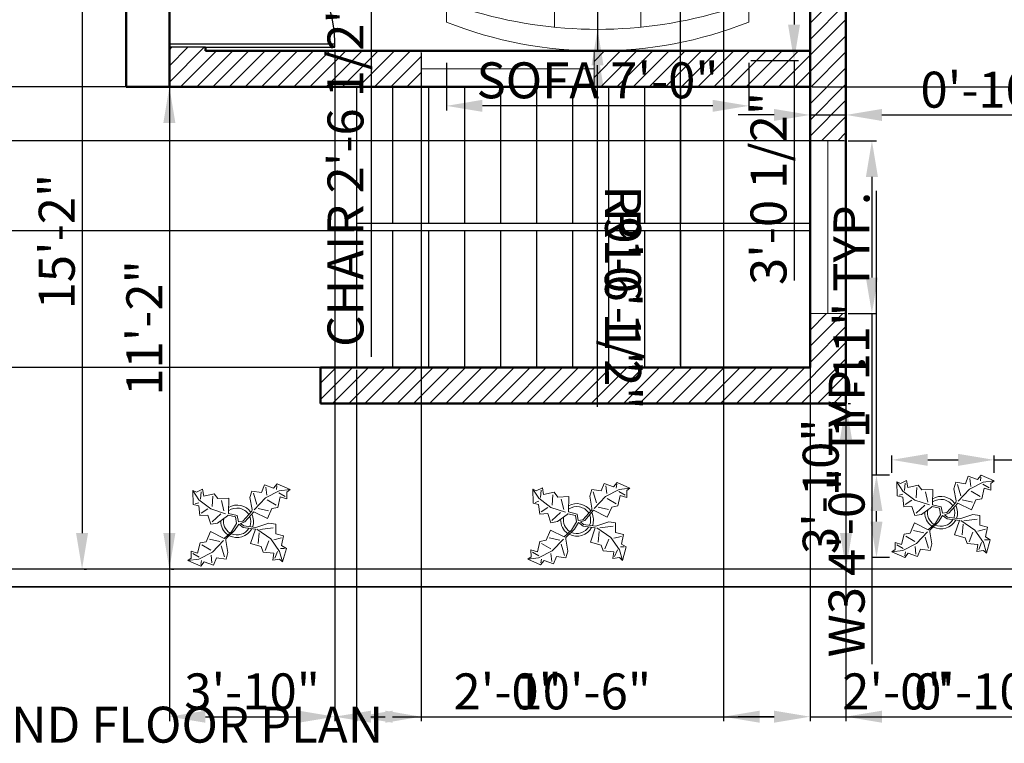
# Model space of a CAD drawing. Units: inches. Extents: x 2206 to 2843, y 1750 to 2489.
# Tile 2 of 8: x 2428 to 2702, y 1751 to 1953. Entities that reach past the tile are written whole.
import ezdxf

# ---------------------------------------------------------------- set-up
doc = ezdxf.new("R2010")
doc.units = ezdxf.units.IN
for name, color, linetype, lineweight in [('A-ANNO-DIMS', 2, 'Continuous', 18), ('A-ANNO-TEXT', 7, 'Continuous', 25), ('A-DOOR', 3, 'Continuous', 25), ('A-FLOR-STRS', 7, 'Continuous', 25), ('A-FURN', 21, 'Continuous', 18), ('A-GLAZ', 4, 'Continuous', 18), ('A-WALL', 7, 'Continuous', 50), ('A-WALL-PATT', 252, 'Continuous', 13), ('C-PROP', 7, 'Continuous', 35), ('L-PLNT', 92, 'Continuous', 18), ('L-SITE-WALL', 8, 'Continuous', 25)]:
    doc.layers.add(name, color=color, linetype=linetype, lineweight=lineweight)
doc.styles.get("Standard").update_dxf_attribs({"font": 'arial.ttf'})
doc.dimstyles.new('ISO-25', dxfattribs={"dimtxt": 10, "dimasz": 10, "dimexe": 1.25, "dimexo": 0.625, "dimtad": 1, "dimdec": 1, "dimlunit": 3, "dimtxsty": 'Standard', "dimcen": 2.5, "dimadec": 0, "dimazin": 0, "dimtfac": 1, "dimtdec": 1, "dimtmove": 0, "dimatfit": 3, "dimfxl": 1, "dimarcsym": 0})

# ---------------------------------------------------------------- blocks, each defined once
blk = doc.blocks.new('Sofa - Roundback 7 ft.')
for p, q in [((-12.00002, -32.4421), (-12.00003, -6.5971)), ((11.99997, -32.4421), (11.99998, -6.5971)), ((-36.000027, -34), (-36.000027, -11.4696)), ((-35.999844, -13.3819), (35.9998, -13.3819)), ((35.99998, -34), (35.99998, -11.4696)), ((-36.000027, -32.4421), (35.99998, -32.4421))]:
    blk.add_line(p, q)
for points in [[(-36.000027, -34), (-42.000027, -34), (-42.000027, -8)], [(41.99998, -8), (41.99998, -34), (35.99998, -34)]]:
    blk.add_lwpolyline(points)
for centre, radius, start, end in [((0, -114.25), 114.25, 68.43141, 111.5686), ((-0.00001, -127.1968), 121.1968, 72.72033, 107.2797)]:
    blk.add_arc(centre, radius, start, end)
blk = doc.blocks.new('Plant - Rubber or Philodendron')
for p, q in [((-16.2005, 11.4774), (-13.9899, 8.1064)), ((-16.2005, 11.4774), (-14.8639, 10.7964)), ((-16.0159, 6.3329), (-16.2005, 11.4774)), ((-14.8639, 10.7964), (-12.6195, 11.8975)), ((-13.3174, 8.325), (-13.0735, 11.0065)), ((-12.6195, 11.8975), (-12.1909, 9.4345)), ((4.6914, 8.8812), (5.3859, 11.2828)), ((5.3859, 11.2828), (8.8871, 10.7908)), ((8.8871, 10.7908), (9.9809, 13.4933)), ((9.9809, 13.4933), (13.3837, 12.301)), ((15.3859, 11.3055), (10.3916, 8.7942)), ((10.5828, 12.6946), (10.8893, 9.7953)), ((13.3837, 12.301), (14.68, 13.9039)), ((14.5816, 13.2037), (14.3848, 11.8033)), ((14.68, 13.9039), (19.3848, 11.8146)), ((19.3848, 11.8146), (15.3859, 11.3055)), ((19.3848, 11.8146), (18.1868, 10.9119)), ((18.1868, 10.9119), (18.1925, 8.4119)), ((-13.9899, 8.1064), (-9.5434, 4.7185)), ((-12.1909, 9.4345), (-8.3829, 10.3)), ((-8.8369, 9.409), (-9.0894, 5.6095)), ((-8.3829, 10.3), (-7.0549, 8.501)), ((-7.0549, 8.501), (-3.0284, 8.6941)), ((-4.8529, 4.012), (-5.7184, 7.82)), ((-3.0284, 8.6941), (-3.0709, 3.1041)), ((4.6914, 8.8812), (5.5014, 4.4831)), ((5.9878, 10.4842), (7.1971, 6.3869)), ((10.3916, 8.7942), (6.2847, 4.4028)), ((14.2977, 6.1031), (10.9934, 7.9956)), ((15.7909, 9.1065), (14.8995, 5.3044)), ((15.2875, 10.6053), (17.5907, 9.2105)), ((18.1925, 8.4119), (15.7909, 9.1065)), ((-14.0069, 5.8704), (-16.0159, 6.3329)), ((-15.3434, 6.5514), (-13.9984, 6.9884)), ((-13.5868, 2.2894), (-14.0069, 5.8704)), ((-13.1329, 3.1804), (-10.6614, 4.727)), ((-9.5434, 4.7185), (-4.1917, 2.9888)), ((2.1141, 0.2298), (5.4346, 3.9146)), ((6.1032, 3.6844), (2.8262, -0.031)), ((5.4346, 3.9146), (5.5014, 4.4831)), ((11.1089, 1.1958), (6.1032, 3.6844)), ((7.7005, 4.8881), (11.5025, 3.9967)), ((12.7005, 4.8994), (11.1089, 1.1958)), ((14.8995, 5.3044), (12.7005, 4.8994)), ((-10.6784, 2.491), (-13.5868, 2.2894)), ((-9.5858, -0.8715), (-10.6784, 2.491)), ((-9.1318, 0.0195), (-5.9793, 2.9025)), ((-7.1228, -0.443), (-3.5248, 2.2131)), ((-3.5248, 2.2131), (-3.3011, 2.4355)), ((-3.3011, 2.4355), (-0.5306, 1.7947)), ((-3.0709, 3.1041), (0.0797, 2.3163)), ((-0.5306, 1.7947), (-0.2255, -0.5527)), ((-0.5306, 1.7947), (-0.5306, 1.7947)), ((0.0797, 2.3163), (0.4866, -0.031)), ((0.4866, -0.031), (2.1141, 0.2298)), ((-11.3237, -7.2629), (-9.7321, -3.5593)), ((-9.7321, -3.5593), (-4.7264, -6.0479)), ((-7.1228, -0.443), (-9.5858, -0.8715)), ((-4.0579, -6.2781), (-0.9375, -3.1608)), ((-2.019, -3.6148), (-0.2255, -0.5527)), ((-0.9375, -3.1608), (0.5883, -0.8135)), ((0.5883, -0.8135), (2.2447, -2.0916)), ((2.8262, -0.031), (1.3003, -0.5527)), ((1.3003, -0.5527), (2.4193, -1.4655)), ((2.2447, -2.0916), (6.7108, -2.6626)), ((2.4193, -1.4655), (6.895, -2.1175)), ((4.943, -7.9659), (6.7108, -2.6626)), ((11.6605, -0.5413), (6.895, -2.1175)), ((12.3677, -6.1981), (7.219, -2.6772)), ((8.3544, -2.7453), (13.1973, -2.1704)), ((11.6605, -0.5413), (14.1354, -0.8948)), ((14.1354, -0.8948), (14.1354, -4.4304)), ((-6.3237, -7.2516), (-10.1257, -6.3602)), ((-9.0148, -11.1577), (-4.9047, -6.8122)), ((-2.019, -3.6148), (-4.7264, -6.0479)), ((-4.1246, -6.8466), (-4.0579, -6.2781)), ((-3.3146, -11.2447), (-4.1246, -6.8466)), ((8.125, -4.0768), (7.7715, -7.9659)), ((10.2463, -10.4408), (11.6605, -6.9053)), ((15.5496, -10.7943), (12.3677, -6.1981)), ((16.2567, -5.8446), (13.4283, -6.5517)), ((14.1354, -4.4304), (16.9638, -5.1375)), ((16.9638, -5.1375), (16.2567, -8.673)), ((-16.8157, -10.7754), (-14.4141, -11.4699)), ((-16.8101, -13.2754), (-16.8157, -10.7754)), ((-14.4141, -11.4699), (-13.5228, -7.6679)), ((-13.5228, -7.6679), (-11.3237, -7.2629)), ((-12.921, -8.4665), (-9.6166, -10.359)), ((-4.611, -12.8477), (-5.8203, -8.7504)), ((8.8321, -9.0266), (4.943, -7.9659)), ((9.5392, -11.1479), (8.8321, -9.0266)), ((14.8425, -10.7943), (13.7819, -13.2692)), ((16.6103, -14.6834), (15.5496, -10.7943)), ((17.3174, -9.7337), (15.9032, -9.7337)), ((16.2567, -8.673), (18.0245, -9.7337)), ((18.0245, -9.7337), (16.6103, -14.6834)), ((-18.008, -14.1781), (-16.8101, -13.2754)), ((-18.008, -14.1781), (-14.0091, -13.669)), ((-13.3032, -16.2674), (-18.008, -14.1781)), ((-13.9107, -12.9688), (-16.2139, -11.574)), ((-14.0091, -13.669), (-9.0148, -11.1577)), ((-13.2048, -15.5672), (-13.008, -14.1668)), ((-9.206, -15.0581), (-9.5126, -12.1588)), ((-7.5103, -13.1543), (-8.6042, -15.8568)), ((-4.0092, -13.6463), (-7.5103, -13.1543)), ((-3.3146, -11.2447), (-4.0092, -13.6463)), ((13.4283, -11.5015), (9.5392, -11.1479)), ((13.0748, -13.9763), (13.4283, -11.5015)), ((15.5496, -13.6228), (13.0748, -13.9763)), ((16.6103, -14.6834), (15.5496, -13.6228)), ((-12.0069, -14.6645), (-13.3032, -16.2674)), ((-8.6042, -15.8568), (-12.0069, -14.6645))]:
    blk.add_line(p, q)
for centre, radius, start, end in [((0, 0), 6.1275, 34.37569, 120.1028), ((-0.0601, -0.2075), 5.2461, 33.82192, 124.9414), ((0.0308, 0.1664), 6, 178.6147, 235.1169), ((0.0308, 0.1664), 5, 168.1647, 238.6725), ((-0.2664, 0.1682), 5.2775, 338.4094, 20.03007), ((-0.098, 0.1364), 6.1288, 341.2017, 26.09184), ((-0.0234, 0.3825), 6.1492, 242.5812, 331.2714), ((-0.1102, 0.4886), 5.2883, 247.3711, 327.472)]:
    blk.add_arc(centre, radius, start, end)
blk = doc.blocks.new('*D16')
at = {"layer": 'A-ANNO-DIMS', "color": 0, "lineweight": -2, "transparency": 16777216}
for p, q in [((2470.2, 1933.9), (2470.83, 1933.9)), ((2469.58, 1923.9), (2469.58, 1809.9)), ((2470.2, 1799.9), (2470.83, 1799.9))]:
    blk.add_line(p, q, dxfattribs=at)
at = {"layer": 'A-ANNO-DIMS', "color": 0, "transparency": 16777216}
for points in [[(2467.91, 1923.9), (2471.25, 1923.9), (2469.58, 1933.9)], [(2467.91, 1809.9), (2471.25, 1809.9), (2469.58, 1799.9)]]:
    blk.add_solid(points, dxfattribs=at)
at = {"layer": 'Defpoints', "color": 0, "transparency": 16777216}
for p in [(2469.58, 1933.9), (2469.58, 1799.9), (2469.58, 1799.9)]:
    blk.add_point(p, dxfattribs=at)
at = {"layer": 'A-ANNO-DIMS', "color": 0, "transparency": 16777216, "insert": (2463.93, 1866.9), "char_height": 10, "attachment_point": 5, "rotation": 90}
blk.add_mtext('11\'-2"', dxfattribs=at)
blk = doc.blocks.new('*D18')
at = {"layer": 'A-ANNO-DIMS', "color": 0, "lineweight": -2, "transparency": 16777216}
for p, q in [((2445.95, 1981.9), (2446.57, 1981.9)), ((2445.32, 1971.9), (2445.32, 1809.9)), ((2445.95, 1799.9), (2446.57, 1799.9))]:
    blk.add_line(p, q, dxfattribs=at)
at = {"layer": 'A-ANNO-DIMS', "color": 0, "transparency": 16777216}
for points in [[(2443.65, 1971.9), (2446.99, 1971.9), (2445.32, 1981.9)], [(2443.65, 1809.9), (2446.99, 1809.9), (2445.32, 1799.9)]]:
    blk.add_solid(points, dxfattribs=at)
at = {"layer": 'Defpoints', "color": 0, "transparency": 16777216}
for p in [(2445.32, 1981.9), (2445.32, 1799.9), (2445.32, 1799.9)]:
    blk.add_point(p, dxfattribs=at)
at = {"layer": 'A-ANNO-DIMS', "color": 0, "transparency": 16777216, "insert": (2439.59, 1890.9), "char_height": 10, "attachment_point": 5, "rotation": 90}
blk.add_mtext('15\'-2"', dxfattribs=at)
blk = doc.blocks.new('*D19')
at = {"layer": 'A-ANNO-DIMS', "color": 0, "lineweight": -2, "transparency": 16777216}
for p, q in [((2658.2, 1845.9), (2658.83, 1845.9)), ((2657.58, 1835.9), (2657.58, 1809.9)), ((2658.2, 1799.9), (2658.83, 1799.9))]:
    blk.add_line(p, q, dxfattribs=at)
at = {"layer": 'A-ANNO-DIMS', "color": 0, "transparency": 16777216}
for points in [[(2655.91, 1835.9), (2659.25, 1835.9), (2657.58, 1845.9)], [(2655.91, 1809.9), (2659.25, 1809.9), (2657.58, 1799.9)]]:
    blk.add_solid(points, dxfattribs=at)
at = {"layer": 'Defpoints', "color": 0, "transparency": 16777216}
for p in [(2657.58, 1845.9), (2657.58, 1799.9), (2657.58, 1799.9)]:
    blk.add_point(p, dxfattribs=at)
at = {"layer": 'A-ANNO-DIMS', "color": 0, "transparency": 16777216, "insert": (2651.85, 1822.9), "char_height": 10, "attachment_point": 5, "rotation": 90}
blk.add_mtext('3\'-10"', dxfattribs=at)
blk = doc.blocks.new('WIN-48IN')
for p, q in [((0, 10), (0, 0)), ((48, 10), (48, 0)), ((48, 5), (0, 5))]:
    blk.add_line(p, q)
blk = doc.blocks.new('*D27')
at = {"layer": 'A-ANNO-DIMS', "color": 0, "lineweight": -2, "transparency": 16777216}
for p, q in [((2670.31, 1826.6), (2670.31, 1831.49)), ((2680.31, 1830.24), (2688.72, 1830.24)), ((2698.72, 1826.6), (2698.72, 1831.49)), ((2698.72, 1830.24), (2842.63, 1830.24))]:
    blk.add_line(p, q, dxfattribs=at)
at = {"layer": 'A-ANNO-DIMS', "color": 0, "transparency": 16777216}
for points in [[(2680.31, 1831.91), (2680.31, 1828.57), (2670.31, 1830.24)], [(2688.72, 1831.91), (2688.72, 1828.57), (2698.72, 1830.24)]]:
    blk.add_solid(points, dxfattribs=at)
at = {"layer": 'Defpoints', "color": 0, "transparency": 16777216}
for p in [(2698.72, 1830.24), (2670.31, 1825.98), (2698.72, 1825.98)]:
    blk.add_point(p, dxfattribs=at)
at = {"layer": 'A-ANNO-DIMS', "color": 0, "transparency": 16777216, "insert": (2775.67, 1836.03), "char_height": 10, "attachment_point": 5}
blk.add_mtext('PLANT 2\'-4 1/2" TYP.', dxfattribs=at)
blk = doc.blocks.new('*D28')
at = {"layer": 'A-ANNO-DIMS', "color": 0, "lineweight": -2, "transparency": 16777216}
for p, q in [((2666.05, 1825.98), (2666.05, 1905.01)), ((2669.69, 1825.98), (2664.8, 1825.98)), ((2666.05, 1813.06), (2666.05, 1815.98)), ((2669.69, 1803.06), (2664.8, 1803.06))]:
    blk.add_line(p, q, dxfattribs=at)
at = {"layer": 'A-ANNO-DIMS', "color": 0, "transparency": 16777216}
for points in [[(2664.38, 1815.98), (2667.72, 1815.98), (2666.05, 1825.98)], [(2664.38, 1813.06), (2667.72, 1813.06), (2666.05, 1803.06)]]:
    blk.add_solid(points, dxfattribs=at)
at = {"layer": 'Defpoints', "color": 0, "transparency": 16777216}
for p in [(2666.05, 1825.98), (2670.31, 1825.98), (2670.31, 1803.06)]:
    blk.add_point(p, dxfattribs=at)
at = {"layer": 'A-ANNO-DIMS', "color": 0, "transparency": 16777216, "insert": (2660.4, 1870.5), "char_height": 10, "attachment_point": 5, "rotation": 90}
blk.add_mtext('1\'-11" TYP.', dxfattribs=at)
blk = doc.blocks.new('*D39')
at = {"layer": 'A-ANNO-DIMS', "color": 0, "lineweight": -2, "transparency": 16777216}
for p, q in [((2658.2, 1918.9), (2666.03, 1918.9)), ((2664.78, 1908.9), (2664.78, 1880.9)), ((2658.2, 1870.9), (2666.03, 1870.9)), ((2664.78, 1870.9), (2664.78, 1773.45))]:
    blk.add_line(p, q, dxfattribs=at)
at = {"layer": 'A-ANNO-DIMS', "color": 0, "transparency": 16777216}
for points in [[(2663.11, 1908.9), (2666.45, 1908.9), (2664.78, 1918.9)], [(2663.11, 1880.9), (2666.45, 1880.9), (2664.78, 1870.9)]]:
    blk.add_solid(points, dxfattribs=at)
at = {"layer": 'Defpoints', "color": 0, "transparency": 16777216}
for p in [(2657.58, 1918.9), (2657.58, 1870.9), (2664.78, 1870.9)]:
    blk.add_point(p, dxfattribs=at)
at = {"layer": 'A-ANNO-DIMS', "color": 0, "transparency": 16777216, "insert": (2659.05, 1817.17), "char_height": 10, "attachment_point": 5, "rotation": 90}
blk.add_mtext('W3 4\'-0" TYP.', dxfattribs=at)
blk = doc.blocks.new('*D40')
at = {"layer": 'A-ANNO-DIMS', "color": 0, "lineweight": -2, "transparency": 16777216}
for p, q in [((2637.58, 1926.1), (2627.58, 1926.1)), ((2647.58, 1919.52), (2647.58, 1927.35)), ((2647.58, 1926.1), (2657.58, 1926.1)), ((2657.58, 1919.52), (2657.58, 1927.35)), ((2667.58, 1926.1), (2747.55, 1926.1))]:
    blk.add_line(p, q, dxfattribs=at)
at = {"layer": 'A-ANNO-DIMS', "color": 0, "transparency": 16777216}
for points in [[(2637.58, 1927.77), (2637.58, 1924.43), (2647.58, 1926.1)], [(2667.58, 1927.77), (2667.58, 1924.43), (2657.58, 1926.1)]]:
    blk.add_solid(points, dxfattribs=at)
at = {"layer": 'Defpoints', "color": 0, "transparency": 16777216}
for p in [(2657.58, 1926.1), (2647.58, 1918.9), (2657.58, 1918.9)]:
    blk.add_point(p, dxfattribs=at)
at = {"layer": 'A-ANNO-DIMS', "color": 0, "transparency": 16777216, "insert": (2712.57, 1931.83), "char_height": 10, "attachment_point": 5}
blk.add_mtext('0\'-10" TYP.', dxfattribs=at)
blk = doc.blocks.new('*D45')
at = {"layer": 'A-ANNO-DIMS', "color": 0, "lineweight": -2, "transparency": 16777216}
for p, q in [((2529.57, 2032.2), (2524.36, 2032.2)), ((2525.61, 2022.2), (2525.61, 2011.61)), ((2529.57, 2001.61), (2524.36, 2001.61)), ((2525.61, 2001.61), (2525.61, 1858.87))]:
    blk.add_line(p, q, dxfattribs=at)
at = {"layer": 'A-ANNO-DIMS', "color": 0, "transparency": 16777216}
for points in [[(2523.94, 2022.2), (2527.27, 2022.2), (2525.61, 2032.2)], [(2523.94, 2011.61), (2527.27, 2011.61), (2525.61, 2001.61)]]:
    blk.add_solid(points, dxfattribs=at)
at = {"layer": 'Defpoints', "color": 0, "transparency": 16777216}
for p in [(2530.19, 2032.2), (2525.61, 2001.61), (2530.19, 2001.61)]:
    blk.add_point(p, dxfattribs=at)
at = {"layer": 'A-ANNO-DIMS', "color": 0, "transparency": 16777216, "insert": (2519.81, 1925.24), "char_height": 10, "attachment_point": 5, "rotation": 90}
blk.add_mtext('CHAIR 2\'-6 1/2" TYP.', dxfattribs=at)
blk = doc.blocks.new('*D51')
at = {"layer": 'A-ANNO-DIMS', "color": 0, "lineweight": -2, "transparency": 16777216}
for p, q in [((2546.55, 1940.61), (2546.55, 1927.38)), ((2630.55, 1940.61), (2630.55, 1927.38)), ((2620.55, 1928.63), (2556.55, 1928.63))]:
    blk.add_line(p, q, dxfattribs=at)
at = {"layer": 'A-ANNO-DIMS', "color": 0, "transparency": 16777216}
for points in [[(2556.55, 1930.3), (2556.55, 1926.97), (2546.55, 1928.63)], [(2620.55, 1930.3), (2620.55, 1926.97), (2630.55, 1928.63)]]:
    blk.add_solid(points, dxfattribs=at)
at = {"layer": 'Defpoints', "color": 0, "transparency": 16777216}
for p in [(2546.55, 1941.23), (2630.55, 1941.23), (2546.55, 1928.63)]:
    blk.add_point(p, dxfattribs=at)
at = {"layer": 'A-ANNO-DIMS', "color": 0, "transparency": 16777216, "insert": (2588.55, 1934.43), "char_height": 10, "attachment_point": 5}
blk.add_mtext('SOFA 7\'-0"', dxfattribs=at)
blk = doc.blocks.new('*D52')
at = {"layer": 'A-ANNO-DIMS', "color": 0, "lineweight": -2, "transparency": 16777216}
for p, q in [((2631.17, 1977.9), (2644.4, 1977.9)), ((2643.15, 1967.9), (2643.15, 1951.23)), ((2631.17, 1941.23), (2644.4, 1941.23)), ((2643.15, 1941.23), (2643.15, 1880.11))]:
    blk.add_line(p, q, dxfattribs=at)
at = {"layer": 'A-ANNO-DIMS', "color": 0, "transparency": 16777216}
for points in [[(2641.48, 1967.9), (2644.81, 1967.9), (2643.15, 1977.9)], [(2641.48, 1951.23), (2644.81, 1951.23), (2643.15, 1941.23)]]:
    blk.add_solid(points, dxfattribs=at)
at = {"layer": 'Defpoints', "color": 0, "transparency": 16777216}
for p in [(2630.55, 1977.9), (2630.55, 1941.23), (2643.15, 1941.23)]:
    blk.add_point(p, dxfattribs=at)
at = {"layer": 'A-ANNO-DIMS', "color": 0, "transparency": 16777216, "insert": (2637.35, 1905.67), "char_height": 10, "attachment_point": 5, "rotation": 90}
blk.add_mtext('3\'-0 1/2"', dxfattribs=at)
blk = doc.blocks.new('*D59')
at = {"layer": 'A-ANNO-DIMS', "color": 0, "lineweight": -2, "transparency": 16777216}
for p, q in [((2521.58, 1855.27), (2521.58, 1757.6)), ((2647.58, 1855.27), (2647.58, 1757.6)), ((2531.58, 1758.85), (2637.58, 1758.85))]:
    blk.add_line(p, q, dxfattribs=at)
at = {"layer": 'A-ANNO-DIMS', "color": 0, "transparency": 16777216}
for points in [[(2531.58, 1760.52), (2531.58, 1757.18), (2521.58, 1758.85)], [(2637.58, 1760.52), (2637.58, 1757.18), (2647.58, 1758.85)]]:
    blk.add_solid(points, dxfattribs=at)
at = {"layer": 'Defpoints', "color": 0, "transparency": 16777216}
for p in [(2521.58, 1855.9), (2647.58, 1855.9), (2647.58, 1758.85)]:
    blk.add_point(p, dxfattribs=at)
at = {"layer": 'A-ANNO-DIMS', "color": 0, "transparency": 16777216, "insert": (2584.58, 1764.58), "char_height": 10, "attachment_point": 5}
blk.add_mtext('10\'-6"', dxfattribs=at)
blk = doc.blocks.new('*D60')
at = {"layer": 'A-ANNO-DIMS', "color": 0, "lineweight": -2, "transparency": 16777216}
for p, q in [((2520.95, 1933.9), (2217.28, 1933.9)), ((2218.53, 1865.9), (2218.53, 1923.9)), ((2520.95, 1855.9), (2217.28, 1855.9))]:
    blk.add_line(p, q, dxfattribs=at)
at = {"layer": 'A-ANNO-DIMS', "color": 0, "transparency": 16777216}
for points in [[(2216.86, 1923.9), (2220.2, 1923.9), (2218.53, 1933.9)], [(2216.86, 1865.9), (2220.2, 1865.9), (2218.53, 1855.9)]]:
    blk.add_solid(points, dxfattribs=at)
at = {"layer": 'Defpoints', "color": 0, "transparency": 16777216}
for p in [(2218.53, 1933.9), (2521.58, 1933.9), (2521.58, 1855.9)]:
    blk.add_point(p, dxfattribs=at)
at = {"layer": 'A-ANNO-DIMS', "color": 0, "transparency": 16777216, "insert": (2212.8, 1894.9), "char_height": 10, "attachment_point": 5, "rotation": 90}
blk.add_mtext('6\'-6"', dxfattribs=at)
blk = doc.blocks.new('*D62')
at = {"layer": 'A-ANNO-DIMS', "color": 0, "lineweight": -2, "transparency": 16777216}
for p, q in [((2469.58, 1944.27), (2469.58, 1757.6)), ((2515.58, 1944.27), (2515.58, 1757.6)), ((2479.58, 1758.85), (2505.58, 1758.85))]:
    blk.add_line(p, q, dxfattribs=at)
at = {"layer": 'A-ANNO-DIMS', "color": 0, "transparency": 16777216}
for points in [[(2479.58, 1760.52), (2479.58, 1757.18), (2469.58, 1758.85)], [(2505.58, 1760.52), (2505.58, 1757.18), (2515.58, 1758.85)]]:
    blk.add_solid(points, dxfattribs=at)
at = {"layer": 'Defpoints', "color": 0, "transparency": 16777216}
for p in [(2469.58, 1944.9), (2515.58, 1944.9), (2515.58, 1758.85)]:
    blk.add_point(p, dxfattribs=at)
at = {"layer": 'A-ANNO-DIMS', "color": 0, "transparency": 16777216, "insert": (2492.58, 1764.58), "char_height": 10, "attachment_point": 5}
blk.add_mtext('3\'-10"', dxfattribs=at)
blk = doc.blocks.new('*D63')
at = {"layer": 'A-ANNO-DIMS', "color": 0, "lineweight": -2, "transparency": 16777216}
for p, q in [((2647.58, 2246.27), (2647.58, 1757.6)), ((2657.58, 2246.27), (2657.58, 1757.6)), ((2637.58, 1758.85), (2627.58, 1758.85)), ((2647.58, 1758.85), (2657.58, 1758.85)), ((2667.58, 1758.85), (2713.18, 1758.85))]:
    blk.add_line(p, q, dxfattribs=at)
at = {"layer": 'A-ANNO-DIMS', "color": 0, "transparency": 16777216}
for points in [[(2637.58, 1760.52), (2637.58, 1757.18), (2647.58, 1758.85)], [(2667.58, 1760.52), (2667.58, 1757.18), (2657.58, 1758.85)]]:
    blk.add_solid(points, dxfattribs=at)
at = {"layer": 'Defpoints', "color": 0, "transparency": 16777216}
for p in [(2647.58, 2246.9), (2657.58, 2246.9), (2657.58, 1758.85)]:
    blk.add_point(p, dxfattribs=at)
at = {"layer": 'A-ANNO-DIMS', "color": 0, "transparency": 16777216, "insert": (2695.38, 1764.58), "char_height": 10, "attachment_point": 5}
blk.add_mtext('0\'-10"', dxfattribs=at)
blk = doc.blocks.new('*D69')
at = {"layer": 'A-ANNO-DIMS', "color": 0, "lineweight": -2, "transparency": 16777216}
for p, q in [((2658.2, 1997.9), (2747.88, 1997.9)), ((2746.63, 1987.9), (2746.63, 1943.9)), ((2648.2, 1933.9), (2747.88, 1933.9))]:
    blk.add_line(p, q, dxfattribs=at)
at = {"layer": 'A-ANNO-DIMS', "color": 0, "transparency": 16777216}
for points in [[(2744.96, 1987.9), (2748.3, 1987.9), (2746.63, 1997.9)], [(2744.96, 1943.9), (2748.3, 1943.9), (2746.63, 1933.9)]]:
    blk.add_solid(points, dxfattribs=at)
at = {"layer": 'Defpoints', "color": 0, "transparency": 16777216}
for p in [(2657.58, 1997.9), (2647.58, 1933.9), (2746.63, 1933.9)]:
    blk.add_point(p, dxfattribs=at)
at = {"layer": 'A-ANNO-DIMS', "color": 0, "transparency": 16777216, "insert": (2740.92, 1965.9), "char_height": 10, "attachment_point": 5, "rotation": 90}
blk.add_mtext('5\'-4"', dxfattribs=at)
blk = doc.blocks.new('*D70')
at = {"layer": 'A-ANNO-DIMS', "color": 0, "lineweight": -2, "transparency": 16777216}
for p, q in [((2515.58, 1944.27), (2515.58, 1757.6)), ((2539.58, 1943.27), (2539.58, 1757.6)), ((2525.58, 1758.85), (2529.58, 1758.85)), ((2539.58, 1758.85), (2577.58, 1758.85))]:
    blk.add_line(p, q, dxfattribs=at)
at = {"layer": 'A-ANNO-DIMS', "color": 0, "transparency": 16777216}
for points in [[(2525.58, 1760.52), (2525.58, 1757.18), (2515.58, 1758.85)], [(2529.58, 1760.52), (2529.58, 1757.18), (2539.58, 1758.85)]]:
    blk.add_solid(points, dxfattribs=at)
at = {"layer": 'Defpoints', "color": 0, "transparency": 16777216}
for p in [(2515.58, 1944.9), (2539.58, 1943.9), (2539.58, 1758.85)]:
    blk.add_point(p, dxfattribs=at)
at = {"layer": 'A-ANNO-DIMS', "color": 0, "transparency": 16777216, "insert": (2563.58, 1764.58), "char_height": 10, "attachment_point": 5}
blk.add_mtext('2\'-0"', dxfattribs=at)
blk = doc.blocks.new('*D71')
at = {"layer": 'A-ANNO-DIMS', "color": 0, "lineweight": -2, "transparency": 16777216}
for p, q in [((2218.53, 1943.9), (2218.53, 1980.79)), ((2646.95, 1933.9), (2217.28, 1933.9)), ((2218.53, 1918.9), (2218.53, 1933.9)), ((2656.95, 1918.9), (2217.28, 1918.9)), ((2218.53, 1908.9), (2218.53, 1898.9))]:
    blk.add_line(p, q, dxfattribs=at)
at = {"layer": 'A-ANNO-DIMS', "color": 0, "transparency": 16777216}
for points in [[(2216.86, 1943.9), (2220.2, 1943.9), (2218.53, 1933.9)], [(2216.86, 1908.9), (2220.2, 1908.9), (2218.53, 1918.9)]]:
    blk.add_solid(points, dxfattribs=at)
at = {"layer": 'Defpoints', "color": 0, "transparency": 16777216}
for p in [(2218.53, 1933.9), (2647.58, 1933.9), (2657.58, 1918.9)]:
    blk.add_point(p, dxfattribs=at)
at = {"layer": 'A-ANNO-DIMS', "color": 0, "transparency": 16777216, "insert": (2212.8, 1967.34), "char_height": 10, "attachment_point": 5, "rotation": 90}
blk.add_mtext('1\'-3"', dxfattribs=at)
blk = doc.blocks.new('*D74')
at = {"layer": 'A-ANNO-DIMS', "color": 0, "lineweight": -2, "transparency": 16777216}
for p, q in [((2611.58, 1856.52), (2611.58, 2432.2)), ((2647.58, 1856.52), (2647.58, 2432.2)), ((2621.58, 2430.95), (2637.58, 2430.95))]:
    blk.add_line(p, q, dxfattribs=at)
at = {"layer": 'A-ANNO-DIMS', "color": 0, "transparency": 16777216}
for points in [[(2621.58, 2432.62), (2621.58, 2429.28), (2611.58, 2430.95)], [(2637.58, 2432.62), (2637.58, 2429.28), (2647.58, 2430.95)]]:
    blk.add_solid(points, dxfattribs=at)
at = {"layer": 'Defpoints', "color": 0, "transparency": 16777216}
for p in [(2647.58, 2430.95), (2611.58, 1855.9), (2647.58, 1855.9)]:
    blk.add_point(p, dxfattribs=at)
at = {"layer": 'A-ANNO-DIMS', "color": 0, "transparency": 16777216, "insert": (2629.58, 2436.68), "char_height": 10, "attachment_point": 5}
blk.add_mtext('3\'-0"', dxfattribs=at)
blk = doc.blocks.new('*D75')
at = {"layer": 'A-ANNO-DIMS', "color": 0, "lineweight": -2, "transparency": 16777216}
for p, q in [((2520.95, 1893.9), (2217.28, 1893.9)), ((2218.53, 1883.9), (2218.53, 1865.9)), ((2520.95, 1855.9), (2217.28, 1855.9))]:
    blk.add_line(p, q, dxfattribs=at)
at = {"layer": 'A-ANNO-DIMS', "color": 0, "transparency": 16777216}
for points in [[(2216.86, 1883.9), (2220.2, 1883.9), (2218.53, 1893.9)], [(2216.86, 1865.9), (2220.2, 1865.9), (2218.53, 1855.9)]]:
    blk.add_solid(points, dxfattribs=at)
at = {"layer": 'Defpoints', "color": 0, "transparency": 16777216}
for p in [(2521.58, 1893.9), (2218.53, 1855.9), (2521.58, 1855.9)]:
    blk.add_point(p, dxfattribs=at)
at = {"layer": 'A-ANNO-DIMS', "color": 0, "transparency": 16777216, "insert": (2212.8, 1874.9), "char_height": 10, "attachment_point": 5, "rotation": 90}
blk.add_mtext('3\'-2"', dxfattribs=at)
blk = doc.blocks.new('*D77')
at = {"layer": 'A-ANNO-DIMS', "color": 0, "lineweight": -2, "transparency": 16777216}
for p, q in [((2623.58, 2204.27), (2623.58, 1757.6)), ((2647.58, 2204.27), (2647.58, 1757.6)), ((2633.58, 1758.85), (2637.58, 1758.85)), ((2647.58, 1758.85), (2685.58, 1758.85))]:
    blk.add_line(p, q, dxfattribs=at)
at = {"layer": 'A-ANNO-DIMS', "color": 0, "transparency": 16777216}
for points in [[(2633.58, 1760.52), (2633.58, 1757.18), (2623.58, 1758.85)], [(2637.58, 1760.52), (2637.58, 1757.18), (2647.58, 1758.85)]]:
    blk.add_solid(points, dxfattribs=at)
at = {"layer": 'Defpoints', "color": 0, "transparency": 16777216}
for p in [(2623.58, 2204.9), (2647.58, 2204.9), (2647.58, 1758.85)]:
    blk.add_point(p, dxfattribs=at)
at = {"layer": 'A-ANNO-DIMS', "color": 0, "transparency": 16777216, "insert": (2671.58, 1764.58), "char_height": 10, "attachment_point": 5}
blk.add_mtext('2\'-0"', dxfattribs=at)
blk = doc.blocks.new('*D80')
at = {"layer": 'A-ANNO-DIMS', "color": 0, "lineweight": -2, "transparency": 16777216}
for p, q in [((2588.55, 2071.1), (2588.55, 1949.9)), ((2588.55, 1854.6), (2588.55, 1939.9))]:
    blk.add_line(p, q, dxfattribs=at)
at = {"layer": 'A-ANNO-DIMS', "color": 0, "transparency": 16777216}
blk.add_solid([(2590.21, 1939.9), (2586.88, 1939.9), (2588.55, 1949.9)], dxfattribs=at)
at = {"layer": 'Defpoints', "color": 0, "transparency": 16777216}
for p in [(2588.55, 2071.1), (2588.55, 1949.9)]:
    blk.add_point(p, dxfattribs=at)
at = {"layer": 'A-ANNO-DIMS', "color": 0, "transparency": 16777216, "insert": (2594.28, 1877.18), "char_height": 10, "attachment_point": 5, "rotation": 270.0002}
blk.add_mtext('R10\'-1"', dxfattribs=at)
blk = doc.blocks.new('*D81')
at = {"layer": 'A-ANNO-DIMS', "color": 0, "lineweight": -2, "transparency": 16777216}
for p, q in [((2588.55, 2058.15), (2588.55, 1943.9)), ((2588.55, 1845), (2588.55, 1933.9))]:
    blk.add_line(p, q, dxfattribs=at)
at = {"layer": 'A-ANNO-DIMS', "color": 0, "transparency": 16777216}
blk.add_solid([(2590.21, 1933.9), (2586.88, 1933.9), (2588.55, 1943.9)], dxfattribs=at)
at = {"layer": 'Defpoints', "color": 0, "transparency": 16777216}
for p in [(2588.55, 2058.15), (2588.55, 1943.9)]:
    blk.add_point(p, dxfattribs=at)
at = {"layer": 'A-ANNO-DIMS', "color": 0, "transparency": 16777216, "insert": (2594.34, 1875.35), "char_height": 10, "attachment_point": 5, "rotation": 270.0002}
blk.add_mtext('R9\'-6 1/2"', dxfattribs=at)

msp = doc.modelspace()

# ---------------------------------------------------------------- hatches: boundary and pattern name
at = {"layer": 'A-WALL-PATT'}
h = msp.add_hatch(dxfattribs=at)
h.set_pattern_fill('ANSI31', color=256)
h.paths.add_polyline_path([(2710.58, 2394.9), (2296.58, 2394.9), (2296.58, 2335.9), (2306.58, 2335.9), (2306.58, 2384.9), (2479.58, 2384.9), (2652.58, 2384.9), (2700.58, 2384.9), (2700.58, 2300.9), (2690.58, 2300.9), (2690.58, 2290.9), (2710.58, 2290.9)])
h.paths.add_polyline_path([(2306.58, 2295.9), (2296.58, 2295.9), (2296.58, 2225.9), (2306.58, 2225.9), (2306.58, 2241.9)])
h.paths.add_polyline_path([(2306.58, 2111.9), (2306.58, 2132.9), (2296.58, 2132.9), (2296.58, 2071.9), (2306.58, 2071.9)])
h.paths.add_polyline_path([(2306.58, 2197.9), (2296.58, 2197.9), (2296.58, 2160.9), (2306.58, 2160.9), (2306.58, 2176.9)])
h.paths.add_polyline_path([(2370.58, 1991.9), (2306.58, 1991.9), (2306.58, 2031.9), (2296.58, 2031.9), (2296.58, 1981.9), (2370.58, 1981.9)])
h.paths.add_polyline_path([(2479.58, 2066.9), (2474.58, 2066.9), (2474.58, 1991.9), (2410.58, 1991.9), (2410.58, 1981.9), (2479.58, 1981.9)])
h.paths.add_polyline_path([(2539.58, 1943.9), (2479.58, 1943.9), (2479.58, 1944.9), (2469.58, 1944.9), (2469.58, 1933.9), (2539.58, 1933.9)])
h.paths.add_polyline_path([(2657.58, 1997.9), (2647.58, 1997.9), (2647.58, 1943.9), (2647.58, 1918.9), (2657.58, 1918.9)])
h.paths.add_polyline_path([(2647.58, 1943.9), (2587.58, 1943.9), (2587.58, 1933.9), (2647.58, 1933.9)])
h.paths.add_polyline_path([(2657.58, 2158.4), (2647.58, 2158.4), (2647.58, 2104.9), (2647.58, 2045.9), (2657.58, 2045.9)])
h.paths.add_polyline_path([(2657.58, 2204.89), (2647.58, 2204.89), (2647.58, 2188.4), (2657.58, 2188.4)])
h.paths.add_polyline_path([(2657.58, 2246.9), (2647.58, 2246.9), (2647.58, 2234.9), (2657.58, 2234.9)])
h.paths.add_polyline_path([(2662.58, 2300.9), (2652.58, 2300.9), (2652.58, 2346.22), (2647.58, 2346.22), (2647.58, 2290.9), (2662.58, 2290.9)])
h.paths.add_polyline_path([(2647.58, 2246.9), (2524.58, 2246.9), (2524.58, 2241.9), (2647.58, 2241.9)])
h.paths.add_polyline_path([(2351.58, 2246.9), (2306.58, 2246.9), (2306.58, 2241.9), (2351.58, 2241.9)])
h.paths.add_polyline_path([(2429.58, 2246.9), (2381.58, 2246.9), (2381.58, 2241.9), (2390.58, 2241.9), (2390.58, 2181.9), (2306.58, 2181.9), (2306.58, 2176.9), (2390.58, 2176.9), (2390.58, 2116.9), (2381.58, 2116.9), (2381.58, 2111.9), (2474.58, 2111.9), (2474.58, 2102.9), (2479.58, 2102.9), (2479.58, 2104.9), (2479.58, 2116.9), (2395.58, 2116.9), (2395.58, 2176.9), (2395.58, 2241.9), (2429.58, 2241.9)])
h.paths.add_polyline_path([(2479.58, 2384.9), (2474.58, 2384.9), (2474.58, 2246.9), (2465.58, 2246.9), (2465.58, 2241.9), (2479.58, 2241.9), (2488.58, 2241.9), (2488.58, 2246.9), (2479.58, 2246.9)])
h.paths.add_polyline_path([(2657.58, 1870.9), (2647.58, 1870.9), (2647.58, 1855.9), (2511.58, 1855.9), (2511.58, 1845.9), (2657.58, 1845.9)])

# ---------------------------------------------------------------- linework, layer by layer
at = {"layer": 'A-DOOR'}
for p, q in [((2469.58, 1945.9), (2515.58, 1945.9)), ((2479.58, 1944.9), (2469.58, 1944.9)), ((2479.58, 1944.9), (2515.58, 1944.9))]:
    msp.add_line(p, q, dxfattribs=at)
msp.add_arc((2480.08, 1945.4), 35.5, 359.1931, 90.8069, dxfattribs=at)
at = {"layer": 'A-FLOR-STRS'}
for p, q in [((2521.58, 1933.9), (2521.58, 1855.9)), ((2531.58, 1933.9), (2531.58, 1895.9)), ((2541.58, 1933.9), (2541.58, 1895.9)), ((2551.58, 1933.9), (2551.58, 1895.9)), ((2561.58, 1933.9), (2561.58, 1895.9)), ((2571.58, 1933.9), (2571.58, 1895.9)), ((2581.58, 1933.9), (2581.58, 1895.9)), ((2591.58, 1933.9), (2591.58, 1895.9)), ((2601.58, 1933.9), (2601.58, 1895.9)), ((2611.58, 1933.9), (2611.58, 1895.9)), ((2647.58, 1895.9), (2521.58, 1895.9)), ((2647.58, 1893.9), (2521.58, 1893.9)), ((2531.58, 1893.9), (2531.58, 1855.9)), ((2541.58, 1893.9), (2541.58, 1855.9)), ((2551.58, 1893.9), (2551.58, 1855.9)), ((2561.58, 1893.9), (2561.58, 1855.9)), ((2571.58, 1893.9), (2571.58, 1855.9)), ((2581.58, 1893.9), (2581.58, 1855.9)), ((2591.58, 1893.9), (2591.58, 1855.9)), ((2601.58, 1893.9), (2601.58, 1855.9)), ((2611.58, 1893.9), (2611.58, 1855.9))]:
    msp.add_line(p, q, dxfattribs=at)
at = {"layer": 'A-WALL'}
for p, q in [((2657.58, 2290.9), (2657.58, 1845.9)), ((2647.58, 2104.9), (2647.58, 1943.9)), ((2457.58, 1933.9), (2457.58, 1981.9)), ((2469.58, 1933.9), (2469.58, 1981.9)), ((2479.58, 1943.9), (2479.58, 1944.9)), ((2479.58, 1943.9), (2647.58, 1943.9)), ((2647.58, 1943.9), (2647.58, 1855.9)), ((2457.58, 1933.9), (2647.58, 1933.9)), ((2647.58, 1855.9), (2511.58, 1855.9)), ((2511.58, 1855.9), (2511.58, 1845.9)), ((2657.58, 1845.9), (2511.58, 1845.9))]:
    msp.add_line(p, q, dxfattribs=at)
at = {"layer": 'C-PROP'}
msp.add_line((2710.58, 1794.9), (2254.58, 1794.9), dxfattribs=at)
at = {"layer": 'L-SITE-WALL'}
msp.add_line((2705.58, 1799.9), (2259.58, 1799.9), dxfattribs=at)

# ---------------------------------------------------------------- block references
at = {"layer": 'A-FURN', "rotation": 180}
msp.add_blockref('Sofa - Roundback 7 ft.', (2588.55, 1943.9), dxfattribs=at)
at = {"layer": 'A-GLAZ'}
msp.add_blockref('WIN-48IN', (2539.58, 1933.9), dxfattribs=at)
at = {"layer": 'A-GLAZ', "rotation": 270.0000000000003}
msp.add_blockref('WIN-48IN', (2647.58, 1918.9), dxfattribs=at)
at = {"layer": 'L-PLNT', "xscale": 0.7595985084536371, "yscale": 0.7595985084536371, "zscale": 0.7595985084536371}
for p in [(2683.99, 1815.42), (2488.39, 1813.01), (2582.83, 1813.41)]:
    msp.add_blockref('Plant - Rubber or Philodendron', p, dxfattribs=at)

# ---------------------------------------------------------------- texts
at = {"layer": 'A-ANNO-TEXT', "insert": (2387.56, 1761.63), "char_height": 10, "attachment_point": 1}
msp.add_mtext_dynamic_manual_height_columns('{\\fArial|b1|i0|c0|p34;GROUND FLOOR PLAN}', width=169.89, gutter_width=12.5, heights=[0], dxfattribs=at)

# ---------------------------------------------------------------- dimensions: what is measured, and where the dimension line sits
at = {"layer": 'A-ANNO-DIMS'}
for base, p1, p2, picture, middle in [((2647.58, 2430.95), (2611.58, 1855.9), (2647.58, 1855.9), '*D74', (2629.58, 2436.68)), ((2657.58, 1758.85), (2647.58, 2246.9), (2657.58, 2246.9), '*D63', (2695.38, 1764.58)), ((2647.58, 1758.85), (2623.58, 2204.9), (2647.58, 2204.9), '*D77', (2671.58, 1764.58)), ((2515.58, 1758.85), (2469.58, 1944.9), (2515.58, 1944.9), '*D62', (2492.58, 1764.58)), ((2539.58, 1758.85), (2515.58, 1944.9), (2539.58, 1943.9), '*D70', (2563.58, 1764.58)), ((2647.58, 1758.85), (2521.58, 1855.9), (2647.58, 1855.9), '*D59', (2584.58, 1764.58))]:
    dim = msp.add_linear_dim(base=base, p1=p1, p2=p2, dimstyle='ISO-25', override={"dimdec": 1, "dimlfac": 1, "dimrnd": 0, "dimzin": 1, "dimdsep": 46, "dimlunit": 4, "dimfrac": 2}, dxfattribs=at)
    dim.commit()
    dim.dimension.update_dxf_attribs({"geometry": picture, "text_midpoint": middle})
for center, mpoint, picture, middle in [((2588.55, 2071.1), (2588.55, 1949.9), '*D80', (2588.55, 1877.18)), ((2588.547664, 2058.149218), (2588.548, 1943.899218), '*D81', (2588.5482016, 1875.349218))]:
    dim = msp.add_radius_dim(center=center, mpoint=mpoint, dimstyle='ISO-25', override={"dimdec": 1, "dimlfac": 1, "dimrnd": 0, "dimzin": 1, "dimdsep": 46, "dimlunit": 4, "dimfrac": 2}, dxfattribs=at)
    dim.commit()
    dim.dimension.update_dxf_attribs({"geometry": picture, "text_midpoint": middle, "dimtype": 164})
for base, p1, p2, angle, text, picture, middle in [((2525.61, 2001.61), (2530.19, 2032.2), (2530.19, 2001.61), 270, 'CHAIR <> TYP.', '*D45', (2519.81, 1925.24)), ((2546.55, 1928.63), (2630.55, 1941.23), (2546.55, 1941.23), 180, 'SOFA <>', '*D51', (2588.55, 1934.43)), ((2664.78, 1870.9), (2657.58, 1918.9), (2657.58, 1870.9), 270, 'W3 <> TYP.', '*D39', (2659.05, 1817.17)), ((2666.05, 1825.98), (2670.31, 1803.06), (2670.31, 1825.98), 90, '<> TYP.', '*D28', (2660.4, 1870.5))]:
    dim = msp.add_linear_dim(base=base, p1=p1, p2=p2, angle=angle, text=text, dimstyle='ISO-25', override={"dimdec": 1, "dimlfac": 1, "dimrnd": 0, "dimzin": 1, "dimdsep": 46, "dimlunit": 4, "dimfrac": 2}, dxfattribs=at)
    dim.commit()
    dim.dimension.update_dxf_attribs({"geometry": picture, "text_midpoint": middle})
for base, p1, p2, angle, override, picture, middle in [((2746.63, 1933.9), (2657.58, 1997.9), (2647.58, 1933.9), 90, {"dimdec": 1, "dimlfac": 1, "dimrnd": 0, "dimzin": 1, "dimdsep": 46, "dimlunit": 4, "dimfrac": 2}, '*D69', (2740.92, 1965.9)), ((2218.53, 1933.9), (2657.58, 1918.9), (2647.58, 1933.9), 90, {"dimdec": 1, "dimlfac": 1, "dimrnd": 0, "dimzin": 1, "dimdsep": 46, "dimlunit": 4, "dimfrac": 2}, '*D71', (2212.8, 1967.34)), ((2445.32, 1799.9), (2445.32, 1981.9), (2445.32, 1799.9), 90, {"dimclrd": 0, "dimclre": 0, "dimclrt": 0}, '*D18', (2439.59, 1890.9)), ((2643.15, 1941.23), (2630.55, 1977.9), (2630.55, 1941.23), 270, {"dimdec": 1, "dimlfac": 1, "dimrnd": 0, "dimzin": 1, "dimdsep": 46, "dimlunit": 4, "dimfrac": 2}, '*D52', (2637.35, 1905.67)), ((2218.53, 1933.9), (2521.58, 1855.9), (2521.58, 1933.9), 90, {"dimdec": 1, "dimlfac": 1, "dimrnd": 0, "dimzin": 1, "dimdsep": 46, "dimlunit": 4, "dimfrac": 2}, '*D60', (2212.8, 1894.9)), ((2469.58, 1799.9), (2469.58, 1933.9), (2469.58, 1799.9), 90, {"dimclrd": 0, "dimclre": 0, "dimclrt": 0}, '*D16', (2463.93, 1866.9)), ((2218.53, 1855.9), (2521.58, 1893.9), (2521.58, 1855.9), 90, {"dimdec": 1, "dimlfac": 1, "dimrnd": 0, "dimzin": 1, "dimdsep": 46, "dimlunit": 4, "dimfrac": 2}, '*D75', (2212.8, 1874.9)), ((2657.58, 1799.9), (2657.58, 1845.9), (2657.58, 1799.9), 90, {"dimclrd": 0, "dimclre": 0, "dimclrt": 0}, '*D19', (2651.85, 1822.9))]:
    dim = msp.add_linear_dim(base=base, p1=p1, p2=p2, angle=angle, dimstyle='ISO-25', override=override, dxfattribs=at)
    dim.commit()
    dim.dimension.update_dxf_attribs({"geometry": picture, "text_midpoint": middle})
for base, p1, p2, text, picture, middle in [((2657.58, 1926.1), (2647.58, 1918.9), (2657.58, 1918.9), '<> TYP.', '*D40', (2712.57, 1931.83)), ((2698.72, 1830.24), (2670.31, 1825.98), (2698.72, 1825.98), 'PLANT <> TYP.', '*D27', (2775.67, 1836.03))]:
    dim = msp.add_linear_dim(base=base, p1=p1, p2=p2, text=text, dimstyle='ISO-25', override={"dimdec": 1, "dimlfac": 1, "dimrnd": 0, "dimzin": 1, "dimdsep": 46, "dimlunit": 4, "dimfrac": 2}, dxfattribs=at)
    dim.commit()
    dim.dimension.update_dxf_attribs({"geometry": picture, "text_midpoint": middle})

doc.saveas('drawing.dxf')
